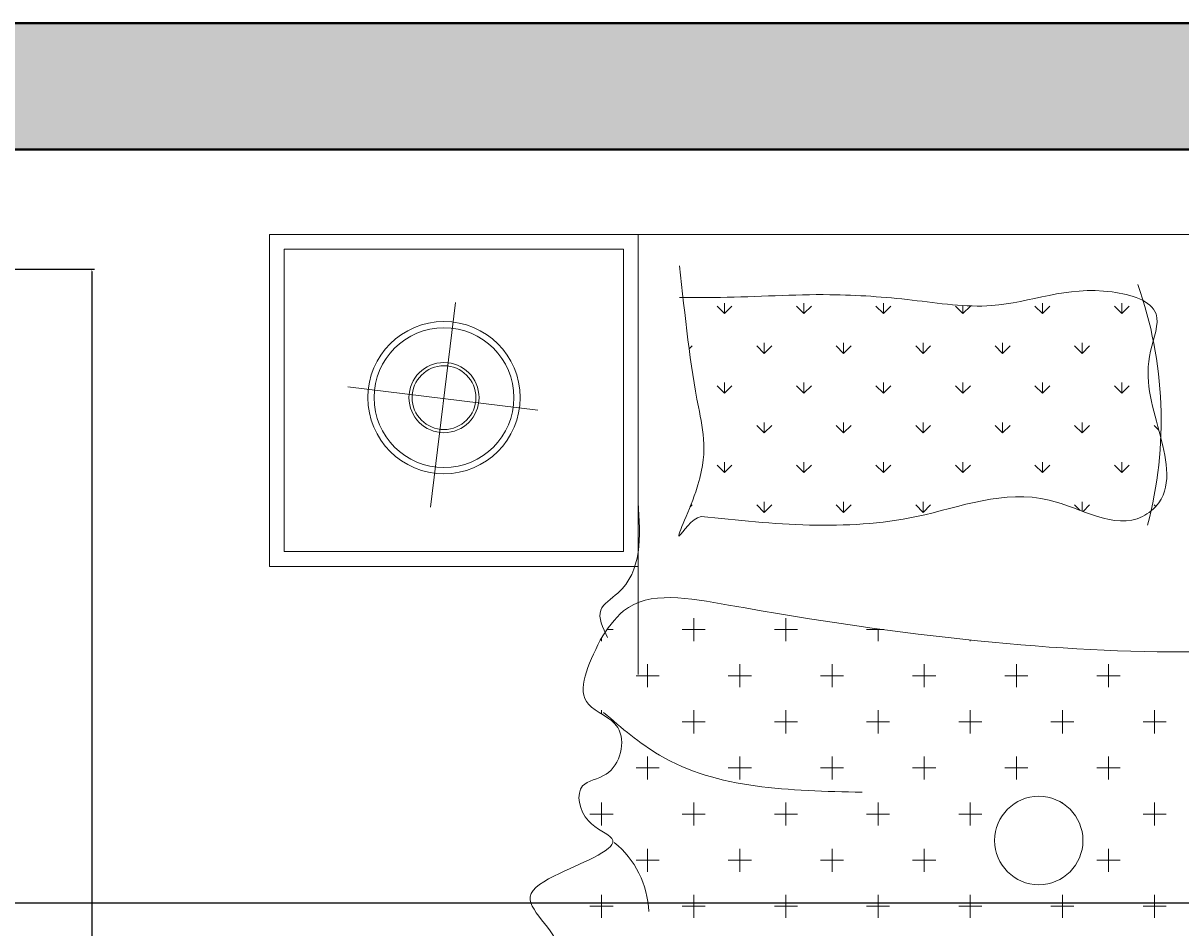
# Model space of a CAD drawing. Units: inches. Extents: x 2330 to 3943, y 1763 to 3461.
# Tile 36 of 40: x 3281 to 3364, y 3098 to 3163. Entities that reach past the tile are written whole.
import ezdxf

# ---------------------------------------------------------------- set-up
doc = ezdxf.new("R2010")
doc.units = ezdxf.units.IN
for name, color, linetype, lineweight in [('A-ANNO-DIMS', 2, 'Continuous', 18), ('A-FURN', 8, 'Continuous', 13), ('A-WALL', 7, 'Continuous', 40), ('A-WALL-PATT', 252, 'Continuous', 13)]:
    doc.layers.add(name, color=color, linetype=linetype, lineweight=lineweight)
doc.styles.get("Standard").update_dxf_attribs({"font": 'arial.ttf'})
doc.dimstyles.get("Standard").update_dxf_attribs({"dimtxt": 0.18, "dimasz": 0.18, "dimexe": 0.18, "dimexo": 0.0625, "dimgap": 0.09, "dimtad": 0, "dimtih": 1, "dimtoh": 1, "dimdec": 4, "dimzin": 0, "dimdsep": 46, "dimtxsty": 'Standard', "dimcen": 0.09, "dimadec": 0, "dimazin": 0, "dimtfac": 1, "dimtdec": 4, "dimtofl": 0, "dimtmove": 0, "dimatfit": 3, "dimfxl": 1, "dimtolj": 1, "dimtzin": 0, "dimarcsym": 0})

# ---------------------------------------------------------------- blocks, each defined once
blk = doc.blocks.new('A$C200C7901')
for p, q in [((0, 1.8834), (0, 2.3334)), ((0.5, 2.3334), (0, 2.3334)), ((0.5, 2.3334), (0.5, 1.7369)), ((0.5, 2.3334), (0.5, 1.7369)), ((0.5, 2.3334), (2, 2.3334)), ((0.9943, 2.1721), (0.9842, 2.1822)), ((0.9943, 2.1721), (0.9842, 2.1822)), ((0.9943, 2.0643), (0.9842, 2.0744)), ((0.9943, 2.0643), (0.9842, 2.0744)), ((1.206, 2.0681), (1.1997, 2.0744)), ((1.206, 2.0681), (1.1997, 2.0744)), ((0.5701, 1.9635), (0.5733, 1.9666)), ((0.5701, 1.9635), (0.5733, 1.9666)), ((1.2019, 1.9645), (1.1997, 1.9666)), ((1.2019, 1.9645), (1.1997, 1.9666)), ((0.5, 1.8834), (0, 1.8834)), ((0.458, 1.7977), (0.466, 1.7977)), ((0.458, 1.7977), (0.466, 1.7977)), ((0.4504, 1.782), (0.4504, 1.7863)), ((0.4504, 1.782), (0.4504, 1.7863)), ((1.1379, 1.7195), (1.1379, 1.7508)), ((1.1222, 1.7352), (1.1535, 1.7352)), ((0.4504, 1.6834), (0.4504, 1.6883)), ((0.4504, 1.6834), (0.4504, 1.6883)), ((0.4656, 1.6727), (0.466, 1.6727)), ((0.4656, 1.6727), (0.466, 1.6727)), ((0.5597, 1.6727), (0.591, 1.6727)), ((0.5597, 1.6727), (0.591, 1.6727)), ((1.0129, 1.5945), (1.0129, 1.6258)), ((1.0129, 1.5945), (1.0129, 1.6258)), ((0.4504, 1.532), (0.4504, 1.5633)), ((1.0754, 1.5625), (1.0754, 1.5633)), ((1.0754, 1.5625), (1.0754, 1.5633)), ((0.4347, 1.5477), (0.466, 1.5477)), ((0.6847, 1.5477), (0.716, 1.5477)), ((0.4347, 1.4227), (0.466, 1.4227))]:
    blk.add_line(p, q)
at = {"linetype": 'ByBlock'}
for p, q in [((0.02, 1.9034), (0.02, 2.3134)), ((0.48, 2.3134), (0.02, 2.3134)), ((0.48, 1.9034), (0.48, 2.3134)), ((0.2524, 2.2412), (0.2186, 1.9635)), ((0.6171, 2.2259), (0.607, 2.236)), ((0.6171, 2.2259), (0.607, 2.236)), ((0.6171, 2.2259), (0.6171, 2.2402)), ((0.6171, 2.2259), (0.6171, 2.2402)), ((0.6171, 2.2259), (0.6272, 2.236)), ((0.6171, 2.2259), (0.6272, 2.236)), ((0.7249, 2.2259), (0.7148, 2.236)), ((0.7249, 2.2259), (0.7148, 2.236)), ((0.7249, 2.2259), (0.7249, 2.2402)), ((0.7249, 2.2259), (0.7249, 2.2402)), ((0.7249, 2.2259), (0.735, 2.236)), ((0.7249, 2.2259), (0.735, 2.236)), ((0.8326, 2.2259), (0.8225, 2.236)), ((0.8326, 2.2259), (0.8225, 2.236)), ((0.8326, 2.2259), (0.8326, 2.2402)), ((0.8326, 2.2259), (0.8326, 2.2402)), ((0.8326, 2.2259), (0.8427, 2.236)), ((0.8326, 2.2259), (0.8427, 2.236)), ((0.9404, 2.2259), (0.9303, 2.236)), ((0.9404, 2.2259), (0.9303, 2.236)), ((0.9404, 2.2259), (0.9404, 2.2369)), ((0.9404, 2.2259), (0.9404, 2.2369)), ((0.9404, 2.2259), (0.9505, 2.236)), ((0.9404, 2.2259), (0.9505, 2.236)), ((1.0482, 2.2259), (1.0381, 2.236)), ((1.0482, 2.2259), (1.0381, 2.236)), ((1.0482, 2.2259), (1.0482, 2.2402)), ((1.0482, 2.2259), (1.0482, 2.2402)), ((1.0482, 2.2259), (1.0583, 2.236)), ((1.0482, 2.2259), (1.0583, 2.236)), ((1.1559, 2.2259), (1.1458, 2.236)), ((1.1559, 2.2259), (1.1458, 2.236)), ((1.1559, 2.2259), (1.1559, 2.2402)), ((1.1559, 2.2259), (1.1559, 2.2402)), ((1.1559, 2.2259), (1.166, 2.236)), ((1.1559, 2.2259), (1.166, 2.236)), ((0.671, 2.172), (0.671, 2.1863)), ((0.671, 2.172), (0.671, 2.1863)), ((0.7787, 2.172), (0.7787, 2.1863)), ((0.7787, 2.172), (0.7787, 2.1863)), ((0.8865, 2.172), (0.8865, 2.1863)), ((0.8865, 2.172), (0.8865, 2.1863)), ((0.9943, 2.172), (0.9943, 2.1863)), ((0.9943, 2.172), (0.9943, 2.1863)), ((1.102, 2.172), (1.102, 2.1863)), ((1.102, 2.172), (1.102, 2.1863)), ((0.5692, 2.178), (0.5733, 2.1822)), ((0.5692, 2.178), (0.5733, 2.1822)), ((0.671, 2.1721), (0.6609, 2.1822)), ((0.671, 2.1721), (0.6609, 2.1822)), ((0.671, 2.1721), (0.6811, 2.1822)), ((0.671, 2.1721), (0.6811, 2.1822)), ((0.7787, 2.1721), (0.7686, 2.1822)), ((0.7787, 2.1721), (0.7686, 2.1822)), ((0.7787, 2.1721), (0.7889, 2.1822)), ((0.7787, 2.1721), (0.7889, 2.1822)), ((0.8865, 2.1721), (0.8764, 2.1822)), ((0.8865, 2.1721), (0.8764, 2.1822)), ((0.8865, 2.1721), (0.8966, 2.1822)), ((0.8865, 2.1721), (0.8966, 2.1822)), ((0.9943, 2.1721), (1.0044, 2.1822)), ((0.9943, 2.1721), (1.0044, 2.1822)), ((1.102, 2.1721), (1.0919, 2.1822)), ((1.102, 2.1721), (1.0919, 2.1822)), ((1.102, 2.1721), (1.1121, 2.1822)), ((1.102, 2.1721), (1.1121, 2.1822)), ((0.3641, 2.0951), (0.1061, 2.1268)), ((0.6171, 2.1182), (0.607, 2.1283)), ((0.6171, 2.1182), (0.607, 2.1283)), ((0.6171, 2.1182), (0.6171, 2.1325)), ((0.6171, 2.1182), (0.6171, 2.1325)), ((0.6171, 2.1182), (0.6272, 2.1283)), ((0.6171, 2.1182), (0.6272, 2.1283)), ((0.7249, 2.1182), (0.7148, 2.1283)), ((0.7249, 2.1182), (0.7148, 2.1283)), ((0.7249, 2.1182), (0.7249, 2.1325)), ((0.7249, 2.1182), (0.7249, 2.1325)), ((0.7249, 2.1182), (0.735, 2.1283)), ((0.7249, 2.1182), (0.735, 2.1283)), ((0.8326, 2.1182), (0.8225, 2.1283)), ((0.8326, 2.1182), (0.8225, 2.1283)), ((0.8326, 2.1182), (0.8326, 2.1325)), ((0.8326, 2.1182), (0.8326, 2.1325)), ((0.8326, 2.1182), (0.8427, 2.1283)), ((0.8326, 2.1182), (0.8427, 2.1283)), ((0.9404, 2.1182), (0.9303, 2.1283)), ((0.9404, 2.1182), (0.9303, 2.1283)), ((0.9404, 2.1182), (0.9404, 2.1325)), ((0.9404, 2.1182), (0.9404, 2.1325)), ((0.9404, 2.1182), (0.9505, 2.1283)), ((0.9404, 2.1182), (0.9505, 2.1283)), ((1.0482, 2.1182), (1.0381, 2.1283)), ((1.0482, 2.1182), (1.0381, 2.1283)), ((1.0482, 2.1182), (1.0482, 2.1325)), ((1.0482, 2.1182), (1.0482, 2.1325)), ((1.0482, 2.1182), (1.0583, 2.1283)), ((1.0482, 2.1182), (1.0583, 2.1283)), ((1.1559, 2.1182), (1.1458, 2.1283)), ((1.1559, 2.1182), (1.1458, 2.1283)), ((1.1559, 2.1182), (1.1559, 2.1325)), ((1.1559, 2.1182), (1.1559, 2.1325)), ((1.1559, 2.1182), (1.166, 2.1283)), ((1.1559, 2.1182), (1.166, 2.1283)), ((0.671, 2.0643), (0.6609, 2.0744)), ((0.671, 2.0643), (0.6609, 2.0744)), ((0.671, 2.0643), (0.671, 2.0786)), ((0.671, 2.0643), (0.671, 2.0786)), ((0.671, 2.0643), (0.6811, 2.0744)), ((0.671, 2.0643), (0.6811, 2.0744)), ((0.7787, 2.0643), (0.7686, 2.0744)), ((0.7787, 2.0643), (0.7686, 2.0744)), ((0.7787, 2.0643), (0.7787, 2.0786)), ((0.7787, 2.0643), (0.7787, 2.0786)), ((0.7787, 2.0643), (0.7889, 2.0744)), ((0.7787, 2.0643), (0.7889, 2.0744)), ((0.8865, 2.0643), (0.8764, 2.0744)), ((0.8865, 2.0643), (0.8764, 2.0744)), ((0.8865, 2.0643), (0.8865, 2.0786)), ((0.8865, 2.0643), (0.8865, 2.0786)), ((0.8865, 2.0643), (0.8966, 2.0744)), ((0.8865, 2.0643), (0.8966, 2.0744)), ((0.9943, 2.0643), (0.9943, 2.0786)), ((0.9943, 2.0643), (0.9943, 2.0786)), ((0.9943, 2.0643), (1.0044, 2.0744)), ((0.9943, 2.0643), (1.0044, 2.0744)), ((1.102, 2.0643), (1.0919, 2.0744)), ((1.102, 2.0643), (1.0919, 2.0744)), ((1.102, 2.0643), (1.102, 2.0786)), ((1.102, 2.0643), (1.102, 2.0786)), ((1.102, 2.0643), (1.1121, 2.0744)), ((1.102, 2.0643), (1.1121, 2.0744)), ((0.6171, 2.0104), (0.607, 2.0205)), ((0.6171, 2.0104), (0.607, 2.0205)), ((0.6171, 2.0104), (0.6171, 2.0247)), ((0.6171, 2.0104), (0.6171, 2.0247)), ((0.6171, 2.0104), (0.6272, 2.0205)), ((0.6171, 2.0104), (0.6272, 2.0205)), ((0.7249, 2.0104), (0.7148, 2.0205)), ((0.7249, 2.0104), (0.7148, 2.0205)), ((0.7249, 2.0104), (0.7249, 2.0247)), ((0.7249, 2.0104), (0.7249, 2.0247)), ((0.7249, 2.0104), (0.735, 2.0205)), ((0.7249, 2.0104), (0.735, 2.0205)), ((0.8326, 2.0104), (0.8225, 2.0205)), ((0.8326, 2.0104), (0.8225, 2.0205)), ((0.8326, 2.0104), (0.8326, 2.0247)), ((0.8326, 2.0104), (0.8326, 2.0247)), ((0.8326, 2.0104), (0.8427, 2.0205)), ((0.8326, 2.0104), (0.8427, 2.0205)), ((0.9404, 2.0104), (0.9303, 2.0205)), ((0.9404, 2.0104), (0.9303, 2.0205)), ((0.9404, 2.0104), (0.9404, 2.0247)), ((0.9404, 2.0104), (0.9404, 2.0247)), ((0.9404, 2.0104), (0.9505, 2.0205)), ((0.9404, 2.0104), (0.9505, 2.0205)), ((1.0482, 2.0104), (1.0381, 2.0205)), ((1.0482, 2.0104), (1.0381, 2.0205)), ((1.0482, 2.0104), (1.0482, 2.0247)), ((1.0482, 2.0104), (1.0482, 2.0247)), ((1.0482, 2.0104), (1.0583, 2.0205)), ((1.0482, 2.0104), (1.0583, 2.0205)), ((1.1559, 2.0104), (1.1458, 2.0205)), ((1.1559, 2.0104), (1.1458, 2.0205)), ((1.1559, 2.0104), (1.1559, 2.0247)), ((1.1559, 2.0104), (1.1559, 2.0247)), ((1.1559, 2.0104), (1.166, 2.0205)), ((1.1559, 2.0104), (1.166, 2.0205)), ((0.671, 1.9565), (0.6609, 1.9666)), ((0.671, 1.9565), (0.6609, 1.9666)), ((0.671, 1.9565), (0.671, 1.9708)), ((0.671, 1.9565), (0.671, 1.9708)), ((0.671, 1.9565), (0.6811, 1.9666)), ((0.671, 1.9565), (0.6811, 1.9666)), ((0.7787, 1.9565), (0.7686, 1.9666)), ((0.7787, 1.9565), (0.7686, 1.9666)), ((0.7787, 1.9565), (0.7787, 1.9708)), ((0.7787, 1.9565), (0.7787, 1.9708)), ((0.7787, 1.9565), (0.7889, 1.9666)), ((0.7787, 1.9565), (0.7889, 1.9666)), ((0.8865, 1.9565), (0.8764, 1.9666)), ((0.8865, 1.9565), (0.8764, 1.9666)), ((0.8865, 1.9565), (0.8865, 1.9708)), ((0.8865, 1.9565), (0.8865, 1.9708)), ((0.8865, 1.9565), (0.8966, 1.9666)), ((0.8865, 1.9565), (0.8966, 1.9666)), ((1.0993, 1.9593), (1.0919, 1.9666)), ((1.0993, 1.9593), (1.0919, 1.9666)), ((1.102, 1.9583), (1.102, 1.9708)), ((1.102, 1.9583), (1.102, 1.9708)), ((1.1033, 1.9578), (1.1121, 1.9666)), ((1.1033, 1.9578), (1.1121, 1.9666)), ((0.48, 1.9034), (0.02, 1.9034)), ((0.5754, 1.782), (0.5754, 1.8133)), ((0.5754, 1.782), (0.5754, 1.8133)), ((0.7004, 1.782), (0.7004, 1.8133)), ((0.7004, 1.782), (0.7004, 1.8133)), ((0.5597, 1.7977), (0.591, 1.7977)), ((0.5597, 1.7977), (0.591, 1.7977)), ((0.6847, 1.7977), (0.716, 1.7977)), ((0.6847, 1.7977), (0.716, 1.7977)), ((0.8097, 1.7977), (0.8331, 1.7977)), ((0.8097, 1.7977), (0.8331, 1.7977)), ((0.8254, 1.782), (0.8254, 1.7987)), ((0.8254, 1.782), (0.8254, 1.7987)), ((0.9504, 1.782), (0.9504, 1.7836)), ((0.9504, 1.782), (0.9504, 1.7836)), ((0.5129, 1.7195), (0.5129, 1.7508)), ((0.5129, 1.7195), (0.5129, 1.7508)), ((0.6379, 1.7195), (0.6379, 1.7508)), ((0.6379, 1.7195), (0.6379, 1.7508)), ((0.7629, 1.7195), (0.7629, 1.7508)), ((0.7629, 1.7195), (0.7629, 1.7508)), ((0.8879, 1.7195), (0.8879, 1.7508)), ((0.8879, 1.7195), (0.8879, 1.7508)), ((1.0129, 1.7195), (1.0129, 1.7508)), ((1.0129, 1.7195), (1.0129, 1.7508)), ((1.1379, 1.7195), (1.1379, 1.7508)), ((0.4972, 1.7352), (0.5285, 1.7352)), ((0.4972, 1.7352), (0.5285, 1.7352)), ((0.6222, 1.7352), (0.6535, 1.7352)), ((0.6222, 1.7352), (0.6535, 1.7352)), ((0.7472, 1.7352), (0.7785, 1.7352)), ((0.7472, 1.7352), (0.7785, 1.7352)), ((0.8722, 1.7352), (0.9035, 1.7352)), ((0.8722, 1.7352), (0.9035, 1.7352)), ((0.9972, 1.7352), (1.0285, 1.7352)), ((0.9972, 1.7352), (1.0285, 1.7352)), ((1.1222, 1.7352), (1.1535, 1.7352)), ((0.5754, 1.657), (0.5754, 1.6883)), ((0.5754, 1.657), (0.5754, 1.6883)), ((0.7004, 1.657), (0.7004, 1.6883)), ((0.7004, 1.657), (0.7004, 1.6883)), ((0.8254, 1.657), (0.8254, 1.6883)), ((0.8254, 1.657), (0.8254, 1.6883)), ((0.9504, 1.657), (0.9504, 1.6883)), ((0.9504, 1.657), (0.9504, 1.6883)), ((1.0754, 1.657), (1.0754, 1.6883)), ((1.0754, 1.657), (1.0754, 1.6883)), ((1.2004, 1.657), (1.2004, 1.6883)), ((1.2004, 1.657), (1.2004, 1.6883)), ((0.6847, 1.6727), (0.716, 1.6727)), ((0.6847, 1.6727), (0.716, 1.6727)), ((0.8097, 1.6727), (0.841, 1.6727)), ((0.8097, 1.6727), (0.841, 1.6727)), ((0.9347, 1.6727), (0.966, 1.6727)), ((0.9347, 1.6727), (0.966, 1.6727)), ((1.0597, 1.6727), (1.091, 1.6727)), ((1.0597, 1.6727), (1.091, 1.6727)), ((1.1847, 1.6727), (1.216, 1.6727)), ((1.1847, 1.6727), (1.216, 1.6727)), ((0.5129, 1.5945), (0.5129, 1.6258)), ((0.5129, 1.5945), (0.5129, 1.6258)), ((0.6379, 1.5945), (0.6379, 1.6258)), ((0.6379, 1.5945), (0.6379, 1.6258)), ((0.7629, 1.5945), (0.7629, 1.6258)), ((0.7629, 1.5945), (0.7629, 1.6258)), ((0.8879, 1.5945), (0.8879, 1.6258)), ((0.8879, 1.5945), (0.8879, 1.6258)), ((1.1379, 1.5945), (1.1379, 1.6258)), ((1.1379, 1.5945), (1.1379, 1.6258)), ((0.4972, 1.6102), (0.5285, 1.6102)), ((0.4972, 1.6102), (0.5285, 1.6102)), ((0.6222, 1.6102), (0.6535, 1.6102)), ((0.6222, 1.6102), (0.6535, 1.6102)), ((0.7472, 1.6102), (0.7785, 1.6102)), ((0.7472, 1.6102), (0.7785, 1.6102)), ((0.8722, 1.6102), (0.9035, 1.6102)), ((0.8722, 1.6102), (0.9035, 1.6102)), ((0.9972, 1.6102), (1.0285, 1.6102)), ((0.9972, 1.6102), (1.0285, 1.6102)), ((1.1222, 1.6102), (1.1535, 1.6102)), ((1.1222, 1.6102), (1.1535, 1.6102)), ((0.4504, 1.532), (0.4504, 1.5633)), ((0.5754, 1.532), (0.5754, 1.5633)), ((0.5754, 1.532), (0.5754, 1.5633)), ((0.7004, 1.532), (0.7004, 1.5633)), ((0.7004, 1.532), (0.7004, 1.5633)), ((0.8254, 1.532), (0.8254, 1.5633)), ((0.8254, 1.532), (0.8254, 1.5633)), ((0.9504, 1.532), (0.9504, 1.5633)), ((0.9504, 1.532), (0.9504, 1.5633)), ((1.2004, 1.532), (1.2004, 1.5633)), ((1.2004, 1.532), (1.2004, 1.5633)), ((0.4347, 1.5477), (0.466, 1.5477)), ((0.5597, 1.5477), (0.591, 1.5477)), ((0.5597, 1.5477), (0.591, 1.5477)), ((0.6847, 1.5477), (0.716, 1.5477)), ((0.8097, 1.5477), (0.841, 1.5477)), ((0.8097, 1.5477), (0.841, 1.5477)), ((0.9347, 1.5477), (0.966, 1.5477)), ((0.9347, 1.5477), (0.966, 1.5477)), ((1.1847, 1.5477), (1.216, 1.5477)), ((1.1847, 1.5477), (1.216, 1.5477)), ((0.5129, 1.4695), (0.5129, 1.5008)), ((0.5129, 1.4695), (0.5129, 1.5008)), ((0.6379, 1.4695), (0.6379, 1.5008)), ((0.6379, 1.4695), (0.6379, 1.5008)), ((0.7629, 1.4695), (0.7629, 1.5008)), ((0.7629, 1.4695), (0.7629, 1.5008)), ((0.8879, 1.4695), (0.8879, 1.5008)), ((0.8879, 1.4695), (0.8879, 1.5008)), ((1.1379, 1.4695), (1.1379, 1.5008)), ((1.1379, 1.4695), (1.1379, 1.5008)), ((0.4972, 1.4852), (0.5285, 1.4852)), ((0.4972, 1.4852), (0.5285, 1.4852)), ((0.6222, 1.4852), (0.6535, 1.4852)), ((0.6222, 1.4852), (0.6535, 1.4852)), ((0.7472, 1.4852), (0.7785, 1.4852)), ((0.7472, 1.4852), (0.7785, 1.4852)), ((0.8722, 1.4852), (0.9035, 1.4852)), ((0.8722, 1.4852), (0.9035, 1.4852)), ((1.1222, 1.4852), (1.1535, 1.4852)), ((1.1222, 1.4852), (1.1535, 1.4852)), ((0.4504, 1.407), (0.4504, 1.4383)), ((0.4504, 1.407), (0.4504, 1.4383)), ((0.5754, 1.407), (0.5754, 1.4383)), ((0.5754, 1.407), (0.5754, 1.4383)), ((0.7004, 1.407), (0.7004, 1.4383)), ((0.7004, 1.407), (0.7004, 1.4383)), ((0.8254, 1.407), (0.8254, 1.4383)), ((0.8254, 1.407), (0.8254, 1.4383)), ((0.9504, 1.407), (0.9504, 1.4383)), ((0.9504, 1.407), (0.9504, 1.4383)), ((1.0754, 1.407), (1.0754, 1.4383)), ((1.0754, 1.407), (1.0754, 1.4383)), ((1.2004, 1.407), (1.2004, 1.4383)), ((1.2004, 1.407), (1.2004, 1.4383)), ((0.4347, 1.4227), (0.466, 1.4227)), ((0.5597, 1.4227), (0.591, 1.4227)), ((0.5597, 1.4227), (0.591, 1.4227)), ((0.6847, 1.4227), (0.716, 1.4227)), ((0.6847, 1.4227), (0.716, 1.4227)), ((0.8097, 1.4227), (0.841, 1.4227)), ((0.8097, 1.4227), (0.841, 1.4227)), ((0.9347, 1.4227), (0.966, 1.4227)), ((0.9347, 1.4227), (0.966, 1.4227)), ((1.0597, 1.4227), (1.091, 1.4227)), ((1.0597, 1.4227), (1.091, 1.4227)), ((1.1847, 1.4227), (1.216, 1.4227)), ((1.1847, 1.4227), (1.216, 1.4227))]:
    blk.add_line(p, q, dxfattribs=at)
for radius in [0.1032, 0.0947, 0.0475, 0.0432]:
    blk.add_circle((0.2367, 2.1121), radius, dxfattribs=at)
blk.add_circle((1.0433, 1.5119), 0.0599)
for centre, radius, start, end in [((0.658, 2.0811), 0.5513, 345.0722, 19.5492), ((0.3888, 1.4113), 0.1256, 1.9962, 51.1646)]:
    blk.add_arc(centre, radius, start, end)
blk.add_arc((0.3888, 1.4113), 0.1256, 1.9962, 51.1646, dxfattribs=at)
for points, knots in [([(0.5562, 2.2908), (0.5634, 2.223), (0.5751, 2.1147), (0.6005, 2.0213), (0.5392, 1.8966), (0.5726, 1.9486), (0.5854, 1.951)], [0, 0, 0, 0, 193.119101, 308.278592, 371.468985, 410.593498, 410.593498, 410.593498, 410.593498]), ([(0.5854, 1.951), (0.6835, 1.9407), (0.8425, 1.9242), (1.0374, 2.0054), (1.1564, 1.9255), (1.2274, 1.9841), (1.2052, 2.0751), (1.1815, 2.152), (1.2176, 2.2368), (1.0992, 2.2731), (1.0008, 2.2255), (0.8698, 2.246), (0.7481, 2.2548), (0.6426, 2.2473), (0.5746, 2.2478), (0.5562, 2.2479)], [0, 0, 0, 0, 292.165466, 473.33038, 601.631673, 630.723769, 727.138505, 836.819956, 887.958136, 954.42438, 1118.989809, 1227.016542, 1338.750986, 1487.447361, 1542.751028, 1542.751028, 1542.751028, 1542.751028]), ([(0.4485, 1.7835), (0.4321, 1.7496), (0.4062, 1.6964), (0.49, 1.6713), (0.4719, 1.5969), (0.4123, 1.592), (0.4233, 1.5337), (0.4954, 1.5086), (0.4012, 1.4738), (0.3253, 1.4306), (0.4113, 1.3764), (0.3688, 1.3065), (0.5579, 1.2663), (0.741, 1.4533), (1.1127, 1.1109), (1.4811, 1.2478), (1.7885, 1.3492), (2.0357, 1.1637), (2.0748, 1.2974), (2.0876, 1.349), (2.0192, 1.3805), (2.0564, 1.4298), (2.0588, 1.4846), (1.9759, 1.5349), (2.1004, 1.5845), (2.0397, 1.6519), (1.971, 1.7053), (2.1104, 1.8981), (1.5946, 1.7967), (1.2448, 1.7472), (0.8129, 1.7935), (0.4953, 1.8548), (0.4582, 1.7983), (0.4485, 1.7835)], [0, 0, 0, 0, 88.420092, 139.08588, 204.302936, 239.695496, 287.801042, 327.365471, 412.960499, 463.626286, 552.059846, 584.668336, 662.614915, 940.993281, 1309.926334, 1844.022653, 1996.276242, 2316.43048, 2341.441004, 2404.707416, 2449.463774, 2514.680778, 2538.40571, 2613.031547, 2697.13096, 2760.903931, 2822.692699, 2945.47, 3215.060018, 3725.584917, 4361.974444, 4504.671998, 4555.32777, 4555.32777, 4555.32777, 4555.32777])]:
    blk.add_open_spline(points, degree=3, knots=knots)
for points, knots in [([(0.5, 1.9703), (0.5029, 1.9235), (0.5066, 1.8648), (0.4398, 1.8252), (0.452, 1.8005), (0.4585, 1.7872)], [0, 0, 0, 0, 126.315232, 158.854004, 196.789047, 196.789047, 196.789047, 196.789047]), ([(0.5, 1.9703), (0.5029, 1.9235), (0.5066, 1.8648), (0.4398, 1.8252), (0.452, 1.8005), (0.4585, 1.7872)], [0, 0, 0, 0, 126.315232, 158.854004, 196.789047, 196.789047, 196.789047, 196.789047]), ([(0.4532, 1.6853), (0.4776, 1.6644), (0.574, 1.582), (0.7055, 1.5794), (0.8037, 1.5774)], [0, 0, 0, 0, 94.920667, 374.457292, 374.457292, 374.457292, 374.457292]), ([(0.4532, 1.6853), (0.4776, 1.6644), (0.574, 1.582), (0.7055, 1.5794), (0.8037, 1.5774)], [0, 0, 0, 0, 94.920667, 374.457292, 374.457292, 374.457292, 374.457292])]:
    blk.add_open_spline(points, degree=3, knots=knots, dxfattribs=at)
blk = doc.blocks.new('*D48')
at = {"layer": 'A-ANNO-DIMS', "color": 0, "lineweight": -2, "transparency": 16777216}
for p, q in [((3262.104, 3145.148), (3286.253, 3145.148)), ((3286.073, 3144.968), (3286.073, 3072.539)), ((3286.073, 2999.746), (3286.073, 3072.176)), ((3262.104, 2999.566), (3286.253, 2999.566))]:
    blk.add_line(p, q, dxfattribs=at)
at = {"layer": 'A-ANNO-DIMS', "color": 0, "transparency": 16777216}
for points in [[(3286.043, 3144.968), (3286.103, 3144.968), (3286.073, 3145.148)], [(3286.043, 2999.746), (3286.103, 2999.746), (3286.073, 2999.566)]]:
    blk.add_solid(points, dxfattribs=at)
at = {"layer": 'Defpoints', "color": 0, "transparency": 16777216}
for p in [(3262.041, 3145.148), (3286.073, 3145.148), (3262.041, 2999.566)]:
    blk.add_point(p, dxfattribs=at)
at = {"layer": 'A-ANNO-DIMS', "color": 0, "transparency": 16777216, "insert": (3286.073, 3072.357), "char_height": 0.18, "attachment_point": 5}
blk.add_mtext('\\A1;146', dxfattribs=at)
blk = doc.blocks.new('*D86')
at = {"layer": 'A-ANNO-DIMS', "color": 0, "lineweight": -2, "transparency": 16777216}
for p, q in [((2979.184, 3100.039), (3942.541, 3100.039)), ((3942.361, 3099.859), (3942.361, 3089.719)), ((3942.361, 3079.219), (3942.361, 3089.358)), ((2979.184, 3079.039), (3942.541, 3079.039))]:
    blk.add_line(p, q, dxfattribs=at)
at = {"layer": 'A-ANNO-DIMS', "color": 0, "transparency": 16777216}
for points in [[(3942.331, 3099.859), (3942.391, 3099.859), (3942.361, 3100.039)], [(3942.331, 3079.219), (3942.391, 3079.219), (3942.361, 3079.039)]]:
    blk.add_solid(points, dxfattribs=at)
at = {"layer": 'Defpoints', "color": 0, "transparency": 16777216}
for p in [(2979.122, 3100.039), (2979.122, 3079.039), (3942.361, 3079.039)]:
    blk.add_point(p, dxfattribs=at)
at = {"layer": 'A-ANNO-DIMS', "color": 0, "transparency": 16777216, "insert": (3942.361, 3089.539), "char_height": 0.18, "attachment_point": 5}
blk.add_mtext('\\A1;21', dxfattribs=at)

msp = doc.modelspace()

# ---------------------------------------------------------------- hatches: boundary and pattern name
at = {"layer": 'A-WALL-PATT'}
h = msp.add_hatch(color=256, dxfattribs=at)
h.dxf.hatch_style = 1
h.paths.add_polyline_path([(3455.6605, 3162.6524), (3243.6605, 3162.6524), (3243.6605, 3153.6524), (3270.6605, 3153.6524), (3270.6605, 3114.6524), (3275.6605, 3114.6524), (3275.6605, 3153.6524), (3446.6605, 3153.6524), (3446.6605, 3114.6524), (3455.6605, 3114.6524)])

# ---------------------------------------------------------------- linework, layer by layer
at = {"layer": 'A-WALL'}
for p, q in [((2968.6605, 3162.6524), (3455.6605, 3162.6524)), ((3275.6605, 3153.6524), (3446.6605, 3153.6524))]:
    msp.add_line(p, q, dxfattribs=at)

# ---------------------------------------------------------------- block references
at = {"layer": 'A-FURN', "xscale": 52.5181391560459, "yscale": 52.5181391560459, "zscale": 52.5181391560459}
msp.add_blockref('A$C200C7901', (3298.7219, 3025.0763), dxfattribs=at)

# ---------------------------------------------------------------- dimensions: what is measured, and where the dimension line sits
at = {"layer": 'A-ANNO-DIMS'}
for base, p1, p2, picture, middle in [((3286.0727, 3145.1485), (3262.0412, 2999.5664), (3262.0412, 3145.1485), '*D48', (3286.0727, 3072.3575)), ((3942.361, 3079.0386), (2979.1218, 3100.0386), (2979.1218, 3079.0386), '*D86', (3942.361, 3089.5386))]:
    dim = msp.add_linear_dim(base=base, p1=p1, p2=p2, angle=90, dimstyle='Standard', override={"dimdec": 0, "dimlfac": 1, "dimrnd": 0, "dimzin": 0, "dimdsep": 46, "dimlunit": 2}, dxfattribs=at)
    dim.commit()
    dim.dimension.update_dxf_attribs({"geometry": picture, "text_midpoint": middle})

doc.saveas('drawing.dxf')
